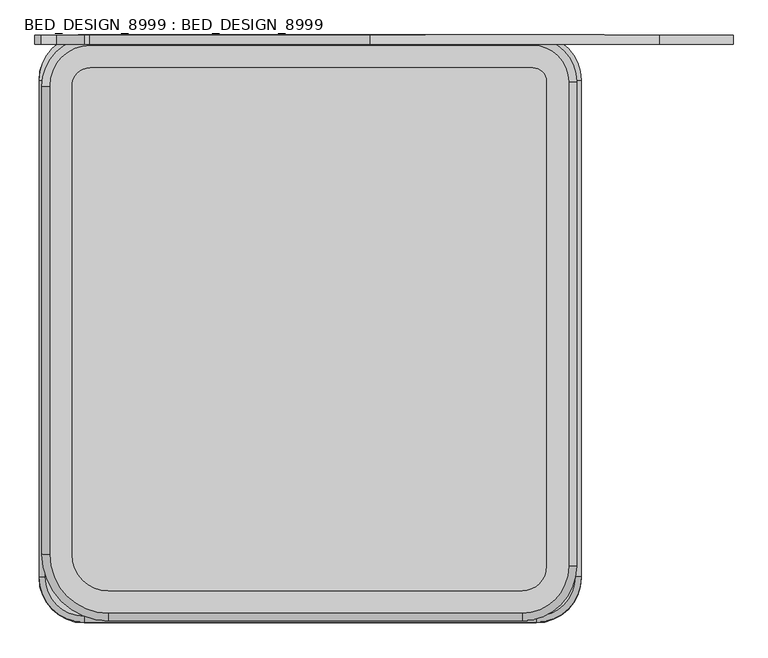
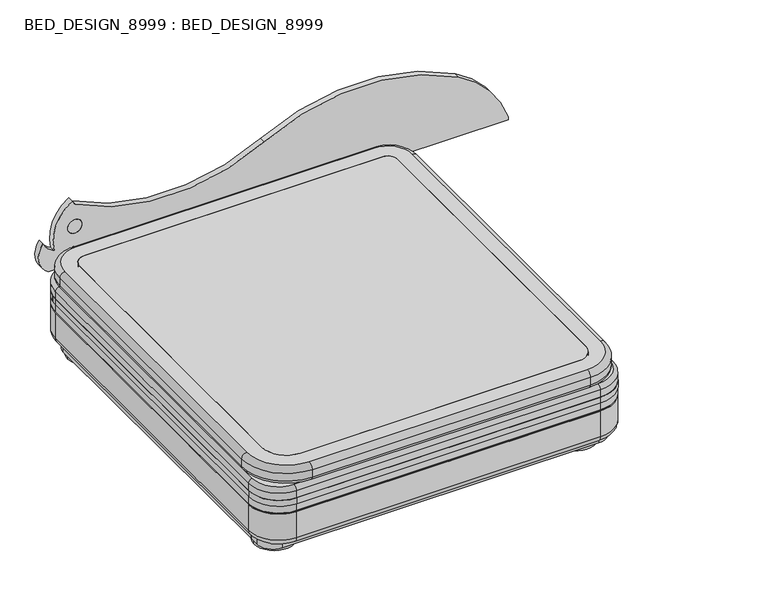
"""IFC4 building model written with IfcOpenShell, lengths in millimetres: furniture geometry, BED_DESIGN_8999 : BED_DESIGN_8999."""

from ifc_helpers import new_model, si_unit, point, frame, frame_2d, origin, origin_with_axes, place, context, project, spatial, polyline, circle_curve, ellipse_curve, trimmed, segment, composite_curve, outline, extrude, source, transform, mapped, element, save
from ifc_brep_helpers import plane_surface, cylinder_surface, revolved_surface, advanced_brep


def bed_design_8999_bed_design_8999_9c973422(model_context):
    return source(origin(), model_context, "Body", "SolidModel", [
        advanced_brep(
        [(550.0, 1945.0, 246.875), (695.0, 1800.0, 246.875), (695.0, 1800.0, 239.375), (550.0, 1945.0, 239.375), (550.0, 1950.0, 350.0), (700.0, 1800.0, 350.0), (700.0, 1800.0, 246.875), (550.0, 1950.0, 246.875), (550.0, 1880.0, 70.0), (630.0, 1800.0, 70.0), (630.0, 1800.0, 370.0), (550.0, 1880.0, 370.0), (550.0, 1950.0, 105.0), (700.0, 1800.0, 105.0), (665.0, 1800.0, 70.0), (550.0, 1915.0, 70.0), (550.0, 1950.0, 239.375), (700.0, 1800.0, 239.375), (-950.0, 1945.0, 239.375), (-950.0, 1945.0, 246.875), (-950.0, 1950.0, 246.875), (-950.0, 1950.0, 350.0), (-950.0, 1880.0, 370.0), (-950.0, 1880.0, 70.0), (-950.0, 1915.0, 70.0), (-950.0, 1950.0, 105.0), (-950.0, 1950.0, 239.375), (-1095.0, 1800.0, 246.875), (-1095.0, 1800.0, 239.375), (-1100.0, 1800.0, 350.0), (-1100.0, 1800.0, 246.875), (-1030.0, 1800.0, 70.0), (-1030.0, 1800.0, 370.0), (-1100.0, 1800.0, 105.0), (-1065.0, 1800.0, 70.0), (-1100.0, 1800.0, 239.375), (-1095.0, 150.0, 239.375), (-1095.0, 150.0, 246.875), (-1100.0, 150.0, 246.875), (-1100.0, 150.0, 350.0), (-1030.0, 150.0, 370.0), (-1030.0, 150.0, 70.0), (-1065.0, 150.0, 70.0), (-1100.0, 150.0, 105.0), (-1100.0, 150.0, 239.375), (-950.0, 5.0, 246.875), (-950.0, 5.0, 239.375), (-950.0, 0.0, 350.0), (-950.0, 0.0, 246.875), (-950.0, 70.0, 70.0), (-950.0, 70.0, 370.0), (-950.0, 0.0, 105.0), (-950.0, 35.0, 70.0), (-950.0, 0.0, 239.375), (550.0, 5.0, 239.375), (550.0, 5.0, 246.875), (550.0, 0.0, 246.875), (550.0, 0.0, 350.0), (550.0, 70.0, 370.0), (550.0, 70.0, 70.0), (550.0, 35.0, 70.0), (550.0, 0.0, 105.0), (550.0, 0.0, 239.375), (695.0, 150.0, 246.875), (695.0, 150.0, 239.375), (700.0, 150.0, 350.0), (700.0, 150.0, 246.875), (630.0, 150.0, 70.0), (630.0, 150.0, 370.0), (700.0, 150.0, 105.0), (665.0, 150.0, 70.0), (700.0, 150.0, 239.375), (-950.0, 20.0, 370.0), (550.0, 20.0, 370.0), (680.0, 150.0, 370.0), (680.0, 1800.0, 370.0), (550.0, 1930.0, 370.0), (-950.0, 1930.0, 370.0), (-1080.0, 1800.0, 370.0), (-1080.0, 150.0, 370.0)],
        [
            (0, 1, circle_curve(frame((550.0, 1800.0, 246.875), z_axis=(0.0, 0.0, -1.0), x_axis=(1.0, 0.0, 0.0)), 145.0)),
            (1, 2),
            (2, 3, circle_curve(frame((550.0, 1800.0, 239.375), z_axis=(0.0, 0.0, 1.0), x_axis=(1.0, 0.0, 0.0)), 145.0)),
            (3, 0),
            (4, 5, circle_curve(frame((550.0, 1800.0, 350.0), z_axis=(0.0, 0.0, -1.0), x_axis=(1.0, 0.0, 0.0)), 150.0)),
            (5, 6),
            (6, 7, circle_curve(frame((550.0, 1800.0, 246.875), z_axis=(0.0, 0.0, 1.0), x_axis=(1.0, 0.0, 0.0)), 150.0)),
            (7, 4),
            (8, 9, circle_curve(frame((550.0, 1800.0, 70.0), z_axis=(0.0, 0.0, -1.0), x_axis=(1.0, 0.0, 0.0)), 80.0)),
            (9, 10),
            (10, 11, circle_curve(frame((550.0, 1800.0, 370.0), z_axis=(0.0, 0.0, 1.0), x_axis=(1.0, 0.0, 0.0)), 80.0)),
            (11, 8),
            (12, 13, circle_curve(frame((550.0, 1800.0, 105.0), z_axis=(0.0, 0.0, -1.0), x_axis=(1.0, 0.0, 0.0)), 150.0)),
            (13, 14, circle_curve(frame((665.0, 1800.0, 105.0), z_axis=(0.0, 1.0, 0.0), x_axis=(1.0, 0.0, 0.0)), 35.0)),
            (14, 15, circle_curve(frame((550.0, 1800.0, 70.0), z_axis=(0.0, 0.0, 1.0), x_axis=(1.0, 0.0, 0.0)), 115.0)),
            (15, 12, circle_curve(frame((550.0, 1915.0, 105.0), z_axis=(1.0, 0.0, 0.0), x_axis=(0.0, 1.0, 0.0)), 35.0)),
            (16, 17, circle_curve(frame((550.0, 1800.0, 239.375), z_axis=(0.0, 0.0, -1.0), x_axis=(1.0, 0.0, 0.0)), 150.0)),
            (17, 13),
            (12, 16),
            (3, 18),
            (18, 19),
            (19, 0),
            (7, 20),
            (20, 21),
            (21, 4),
            (11, 22),
            (22, 23),
            (23, 8),
            (15, 24),
            (24, 25, circle_curve(frame((-950.0, 1915.0, 105.0), z_axis=(1.0, 0.0, 0.0), x_axis=(0.0, 1.0, 0.0)), 35.0)),
            (25, 12),
            (25, 26),
            (26, 16),
            (27, 19, circle_curve(frame((-950.0, 1800.0, 246.875), z_axis=(0.0, 0.0, -1.0), x_axis=(0.0, 1.0, 0.0)), 145.0)),
            (18, 28, circle_curve(frame((-950.0, 1800.0, 239.375), z_axis=(0.0, 0.0, 1.0), x_axis=(0.0, 1.0, 0.0)), 145.0)),
            (28, 27),
            (29, 21, circle_curve(frame((-950.0, 1800.0, 350.0), z_axis=(0.0, 0.0, -1.0), x_axis=(0.0, 1.0, 0.0)), 150.0)),
            (20, 30, circle_curve(frame((-950.0, 1800.0, 246.875), z_axis=(0.0, 0.0, 1.0), x_axis=(0.0, 1.0, 0.0)), 150.0)),
            (30, 29),
            (31, 23, circle_curve(frame((-950.0, 1800.0, 70.0), z_axis=(0.0, 0.0, -1.0), x_axis=(0.0, 1.0, 0.0)), 80.0)),
            (22, 32, circle_curve(frame((-950.0, 1800.0, 370.0), z_axis=(0.0, 0.0, 1.0), x_axis=(0.0, 1.0, 0.0)), 80.0)),
            (32, 31),
            (33, 25, circle_curve(frame((-950.0, 1800.0, 105.0), z_axis=(0.0, 0.0, -1.0), x_axis=(0.0, 1.0, 0.0)), 150.0)),
            (24, 34, circle_curve(frame((-950.0, 1800.0, 70.0), z_axis=(0.0, 0.0, 1.0), x_axis=(0.0, 1.0, 0.0)), 115.0)),
            (34, 33, circle_curve(frame((-1065.0, 1800.0, 105.0), z_axis=(0.0, 1.0, 0.0), x_axis=(-1.0, 0.0, 0.0)), 35.0)),
            (35, 26, circle_curve(frame((-950.0, 1800.0, 239.375), z_axis=(0.0, 0.0, -1.0), x_axis=(0.0, 1.0, 0.0)), 150.0)),
            (33, 35),
            (28, 36),
            (36, 37),
            (37, 27),
            (30, 38),
            (38, 39),
            (39, 29),
            (32, 40),
            (40, 41),
            (41, 31),
            (34, 42),
            (42, 43, circle_curve(frame((-1065.0, 150.0, 105.0), z_axis=(0.0, 1.0, 0.0), x_axis=(-1.0, 0.0, 0.0)), 35.0)),
            (43, 33),
            (43, 44),
            (44, 35),
            (45, 37, circle_curve(frame((-950.0, 150.0, 246.875), z_axis=(0.0, 0.0, -1.0), x_axis=(-1.0, 0.0, 0.0)), 145.0)),
            (36, 46, circle_curve(frame((-950.0, 150.0, 239.375), z_axis=(0.0, 0.0, 1.0), x_axis=(-1.0, 0.0, 0.0)), 145.0)),
            (46, 45),
            (47, 39, circle_curve(frame((-950.0, 150.0, 350.0), z_axis=(0.0, 0.0, -1.0), x_axis=(-1.0, 0.0, 0.0)), 150.0)),
            (38, 48, circle_curve(frame((-950.0, 150.0, 246.875), z_axis=(0.0, 0.0, 1.0), x_axis=(-1.0, 0.0, 0.0)), 150.0)),
            (48, 47),
            (49, 41, circle_curve(frame((-950.0, 150.0, 70.0), z_axis=(0.0, 0.0, -1.0), x_axis=(-1.0, 0.0, 0.0)), 80.0)),
            (40, 50, circle_curve(frame((-950.0, 150.0, 370.0), z_axis=(0.0, 0.0, 1.0), x_axis=(-1.0, 0.0, 0.0)), 80.0)),
            (50, 49),
            (51, 43, circle_curve(frame((-950.0, 150.0, 105.0), z_axis=(0.0, 0.0, -1.0), x_axis=(-1.0, 0.0, 0.0)), 150.0)),
            (42, 52, circle_curve(frame((-950.0, 150.0, 70.0), z_axis=(0.0, 0.0, 1.0), x_axis=(-1.0, 0.0, 0.0)), 115.0)),
            (52, 51, circle_curve(frame((-950.0, 35.0, 105.0), z_axis=(-1.0, 0.0, 0.0), x_axis=(0.0, -1.0, 0.0)), 35.0)),
            (53, 44, circle_curve(frame((-950.0, 150.0, 239.375), z_axis=(0.0, 0.0, -1.0), x_axis=(-1.0, 0.0, 0.0)), 150.0)),
            (51, 53),
            (46, 54),
            (54, 55),
            (55, 45),
            (48, 56),
            (56, 57),
            (57, 47),
            (50, 58),
            (58, 59),
            (59, 49),
            (52, 60),
            (60, 61, circle_curve(frame((550.0, 35.0, 105.0), z_axis=(-1.0, 0.0, 0.0), x_axis=(0.0, -1.0, 0.0)), 35.0)),
            (61, 51),
            (61, 62),
            (62, 53),
            (63, 55, circle_curve(frame((550.0, 150.0, 246.875), z_axis=(0.0, 0.0, -1.0), x_axis=(0.0, -1.0, 0.0)), 145.0)),
            (54, 64, circle_curve(frame((550.0, 150.0, 239.375), z_axis=(0.0, 0.0, 1.0), x_axis=(0.0, -1.0, 0.0)), 145.0)),
            (64, 63),
            (65, 57, circle_curve(frame((550.0, 150.0, 350.0), z_axis=(0.0, 0.0, -1.0), x_axis=(0.0, -1.0, 0.0)), 150.0)),
            (56, 66, circle_curve(frame((550.0, 150.0, 246.875), z_axis=(0.0, 0.0, 1.0), x_axis=(0.0, -1.0, 0.0)), 150.0)),
            (66, 65),
            (67, 59, circle_curve(frame((550.0, 150.0, 70.0), z_axis=(0.0, 0.0, -1.0), x_axis=(0.0, -1.0, 0.0)), 80.0)),
            (58, 68, circle_curve(frame((550.0, 150.0, 370.0), z_axis=(0.0, 0.0, 1.0), x_axis=(0.0, -1.0, 0.0)), 80.0)),
            (68, 67),
            (69, 61, circle_curve(frame((550.0, 150.0, 105.0), z_axis=(0.0, 0.0, -1.0), x_axis=(0.0, -1.0, 0.0)), 150.0)),
            (60, 70, circle_curve(frame((550.0, 150.0, 70.0), z_axis=(0.0, 0.0, 1.0), x_axis=(0.0, -1.0, 0.0)), 115.0)),
            (70, 69, circle_curve(frame((665.0, 150.0, 105.0), z_axis=(0.0, -1.0, 0.0), x_axis=(1.0, 0.0, 0.0)), 35.0)),
            (71, 62, circle_curve(frame((550.0, 150.0, 239.375), z_axis=(0.0, 0.0, -1.0), x_axis=(0.0, -1.0, 0.0)), 150.0)),
            (69, 71),
            (71, 17),
            (2, 64),
            (1, 63),
            (6, 66),
            (5, 65),
            (72, 73),
            (73, 74, circle_curve(frame((550.0, 150.0, 370.0), z_axis=(0.0, 0.0, 1.0), x_axis=(0.0, -1.0, 0.0)), 130.0)),
            (74, 75),
            (75, 76, circle_curve(frame((550.0, 1800.0, 370.0), z_axis=(0.0, 0.0, 1.0), x_axis=(1.0, 0.0, 0.0)), 130.0)),
            (76, 77),
            (77, 78, circle_curve(frame((-950.0, 1800.0, 370.0), z_axis=(0.0, 0.0, 1.0), x_axis=(0.0, 1.0, 0.0)), 130.0)),
            (78, 79),
            (79, 72, circle_curve(frame((-950.0, 150.0, 370.0), z_axis=(0.0, 0.0, 1.0), x_axis=(-1.0, 0.0, 0.0)), 130.0)),
            (10, 68),
            (9, 67),
            (14, 70),
            (13, 69),
            (75, 5, circle_curve(frame((680.0, 1800.0, 350.0), z_axis=(0.0, 1.0, 0.0), x_axis=(1.0, 0.0, 0.0)), 20.0)),
            (4, 76, circle_curve(frame((550.0, 1930.0, 350.0), z_axis=(1.0, 0.0, 0.0), x_axis=(0.0, 1.0, 0.0)), 20.0)),
            (21, 77, circle_curve(frame((-950.0, 1930.0, 350.0), z_axis=(1.0, 0.0, 0.0), x_axis=(0.0, 1.0, 0.0)), 20.0)),
            (29, 78, circle_curve(frame((-1080.0, 1800.0, 350.0), z_axis=(0.0, 1.0, 0.0), x_axis=(-1.0, 0.0, 0.0)), 20.0)),
            (39, 79, circle_curve(frame((-1080.0, 150.0, 350.0), z_axis=(0.0, 1.0, 0.0), x_axis=(-1.0, 0.0, 0.0)), 20.0)),
            (47, 72, circle_curve(frame((-950.0, 20.0, 350.0), z_axis=(-1.0, 0.0, 0.0), x_axis=(0.0, -1.0, 0.0)), 20.0)),
            (57, 73, circle_curve(frame((550.0, 20.0, 350.0), z_axis=(-1.0, 0.0, 0.0), x_axis=(0.0, -1.0, 0.0)), 20.0)),
            (65, 74, circle_curve(frame((680.0, 150.0, 350.0), z_axis=(0.0, -1.0, 0.0), x_axis=(1.0, 0.0, 0.0)), 20.0)),
        ],
        [
            cylinder_surface(frame((550.0, 1800.0, 0.0), z_axis=(0.0, 0.0, 1.0), x_axis=(1.0, 0.0, 0.0)), 145.0),
            cylinder_surface(frame((550.0, 1800.0, 0.0), z_axis=(0.0, 0.0, 1.0), x_axis=(1.0, 0.0, 0.0)), 150.0),
            revolved_surface(polyline([(630.0, 1800.0, 370.0), (630.0, 1800.0, 70.0)]), (550.0, 1800.0, 0.0), (0.0, 0.0, 1.0)),
            revolved_surface(trimmed(ellipse_curve(frame((665.0, 1800.0, 105.0), z_axis=(0.0, -1.0, 0.0), x_axis=(1.0, 0.0, 0.0)), 35.0, 35.0), [point((665.0, 1800.0, 70.0))], [point((700.0, 1800.0, 105.0))], True, "CARTESIAN"), (550.0, 1800.0, 0.0), (0.0, 0.0, 1.0)),
            plane_surface(frame((550.0, 1945.0, 239.375), z_axis=(0.0, 1.0, 0.0), x_axis=(-1.0, 0.0, 0.0))),
            plane_surface(frame((550.0, 1950.0, 246.875), z_axis=(0.0, 1.0, 0.0), x_axis=(-1.0, 0.0, 0.0))),
            plane_surface(frame((550.0, 1880.0, 370.0), z_axis=(0.0, -1.0, 0.0), x_axis=(-1.0, 0.0, 0.0))),
            cylinder_surface(frame((550.0, 1915.0, 105.0), z_axis=(1.0, 0.0, 0.0), x_axis=(0.0, 1.0, 0.0)), 35.0),
            plane_surface(frame((550.0, 1950.0, 105.0), z_axis=(0.0, 1.0, 0.0), x_axis=(-1.0, 0.0, 0.0))),
            cylinder_surface(frame((-950.0, 1800.0, 0.0), z_axis=(0.0, 0.0, 1.0), x_axis=(0.0, 1.0, 0.0)), 145.0),
            cylinder_surface(frame((-950.0, 1800.0, 0.0), z_axis=(0.0, 0.0, 1.0), x_axis=(0.0, 1.0, 0.0)), 150.0),
            revolved_surface(polyline([(-950.0, 1880.0, 370.0), (-950.0, 1880.0, 70.0)]), (-950.0, 1800.0, 0.0), (0.0, 0.0, 1.0)),
            revolved_surface(trimmed(ellipse_curve(frame((-950.0, 1915.0, 105.0), z_axis=(1.0, 0.0, 0.0), x_axis=(0.0, 1.0, 0.0)), 35.0, 35.0), [point((-950.0, 1915.0, 70.0))], [point((-950.0, 1950.0, 105.0))], True, "CARTESIAN"), (-950.0, 1800.0, 0.0), (0.0, 0.0, 1.0)),
            plane_surface(frame((-1095.0, 1800.0, 239.375), z_axis=(-1.0, 0.0, 0.0), x_axis=(0.0, -1.0, 0.0))),
            plane_surface(frame((-1100.0, 1800.0, 246.875), z_axis=(-1.0, 0.0, 0.0), x_axis=(0.0, -1.0, 0.0))),
            plane_surface(frame((-1030.0, 1800.0, 370.0), z_axis=(1.0, 0.0, 0.0), x_axis=(0.0, -1.0, 0.0))),
            cylinder_surface(frame((-1065.0, 1800.0, 105.0), z_axis=(0.0, 1.0, 0.0), x_axis=(-1.0, 0.0, 0.0)), 35.0),
            plane_surface(frame((-1100.0, 1800.0, 105.0), z_axis=(-1.0, 0.0, 0.0), x_axis=(0.0, -1.0, 0.0))),
            cylinder_surface(frame((-950.0, 150.0, 0.0), z_axis=(0.0, 0.0, 1.0), x_axis=(-1.0, 0.0, 0.0)), 145.0),
            cylinder_surface(frame((-950.0, 150.0, 0.0), z_axis=(0.0, 0.0, 1.0), x_axis=(-1.0, 0.0, 0.0)), 150.0),
            revolved_surface(polyline([(-1030.0, 150.0, 370.0), (-1030.0, 150.0, 70.0)]), (-950.0, 150.0, 0.0), (0.0, 0.0, 1.0)),
            revolved_surface(trimmed(ellipse_curve(frame((-1065.0, 150.0, 105.0), z_axis=(0.0, 1.0, 0.0), x_axis=(-1.0, 0.0, 0.0)), 35.0, 35.0), [point((-1065.0, 150.0, 70.0))], [point((-1100.0, 150.0, 105.0))], True, "CARTESIAN"), (-950.0, 150.0, 0.0), (0.0, 0.0, 1.0)),
            plane_surface(frame((-950.0, 5.0, 239.375), z_axis=(0.0, -1.0, 0.0), x_axis=(1.0, 0.0, 0.0))),
            plane_surface(frame((-950.0, 0.0, 246.875), z_axis=(0.0, -1.0, 0.0), x_axis=(1.0, 0.0, 0.0))),
            plane_surface(frame((-950.0, 70.0, 370.0), z_axis=(0.0, 1.0, 0.0), x_axis=(1.0, 0.0, 0.0))),
            cylinder_surface(frame((-950.0, 35.0, 105.0), z_axis=(-1.0, 0.0, 0.0), x_axis=(0.0, -1.0, 0.0)), 35.0),
            plane_surface(frame((-950.0, 0.0, 105.0), z_axis=(0.0, -1.0, 0.0), x_axis=(1.0, 0.0, 0.0))),
            cylinder_surface(frame((550.0, 150.0, 0.0), z_axis=(0.0, 0.0, 1.0), x_axis=(0.0, -1.0, 0.0)), 145.0),
            cylinder_surface(frame((550.0, 150.0, 0.0), z_axis=(0.0, 0.0, 1.0), x_axis=(0.0, -1.0, 0.0)), 150.0),
            revolved_surface(polyline([(550.0, 70.0, 370.0), (550.0, 70.0, 70.0)]), (550.0, 150.0, 0.0), (0.0, 0.0, 1.0)),
            revolved_surface(trimmed(ellipse_curve(frame((550.0, 35.0, 105.0), z_axis=(-1.0, 0.0, 0.0), x_axis=(0.0, -1.0, 0.0)), 35.0, 35.0), [point((550.0, 35.0, 70.0))], [point((550.0, 0.0, 105.0))], True, "CARTESIAN"), (550.0, 150.0, 0.0), (0.0, 0.0, 1.0)),
            plane_surface(frame((700.0, 150.0, 239.375), z_axis=(0.0, 0.0, 1.0), x_axis=(0.0, 1.0, 0.0))),
            plane_surface(frame((695.0, 150.0, 239.375), z_axis=(1.0, 0.0, 0.0), x_axis=(0.0, 1.0, 0.0))),
            plane_surface(frame((695.0, 150.0, 246.875), z_axis=(0.0, 0.0, -1.0), x_axis=(0.0, 1.0, 0.0))),
            plane_surface(frame((700.0, 150.0, 246.875), z_axis=(1.0, 0.0, 0.0), x_axis=(0.0, 1.0, 0.0))),
            plane_surface(frame((680.0, 150.0, 370.0), z_axis=(0.0, 0.0, 1.0), x_axis=(0.0, 1.0, 0.0))),
            plane_surface(frame((630.0, 150.0, 370.0), z_axis=(-1.0, 0.0, 0.0), x_axis=(0.0, 1.0, 0.0))),
            plane_surface(frame((630.0, 150.0, 70.0), z_axis=(0.0, 0.0, -1.0), x_axis=(0.0, 1.0, 0.0))),
            cylinder_surface(frame((665.0, 150.0, 105.0), z_axis=(0.0, -1.0, 0.0), x_axis=(1.0, 0.0, 0.0)), 35.0),
            plane_surface(frame((700.0, 150.0, 105.0), z_axis=(1.0, 0.0, 0.0), x_axis=(0.0, 1.0, 0.0))),
            revolved_surface(trimmed(ellipse_curve(frame((680.0, 1800.0, 350.0), z_axis=(0.0, -1.0, 0.0), x_axis=(1.0, 0.0, 0.0)), 20.0, 20.0), [point((700.0, 1800.0, 350.0))], [point((680.0, 1800.0, 370.0))], True, "CARTESIAN"), (550.0, 1800.0, 0.0), (0.0, 0.0, 1.0)),
            cylinder_surface(frame((550.0, 1930.0, 350.0), z_axis=(1.0, 0.0, 0.0), x_axis=(0.0, 1.0, 0.0)), 20.0),
            revolved_surface(trimmed(ellipse_curve(frame((-950.0, 1930.0, 350.0), z_axis=(1.0, 0.0, 0.0), x_axis=(0.0, 1.0, 0.0)), 20.0, 20.0), [point((-950.0, 1950.0, 350.0))], [point((-950.0, 1930.0, 370.0))], True, "CARTESIAN"), (-950.0, 1800.0, 0.0), (0.0, 0.0, 1.0)),
            cylinder_surface(frame((-1080.0, 1800.0, 350.0), z_axis=(0.0, 1.0, 0.0), x_axis=(-1.0, 0.0, 0.0)), 20.0),
            revolved_surface(trimmed(ellipse_curve(frame((-1080.0, 150.0, 350.0), z_axis=(0.0, 1.0, 0.0), x_axis=(-1.0, 0.0, 0.0)), 20.0, 20.0), [point((-1100.0, 150.0, 350.0))], [point((-1080.0, 150.0, 370.0))], True, "CARTESIAN"), (-950.0, 150.0, 0.0), (0.0, 0.0, 1.0)),
            cylinder_surface(frame((-950.0, 20.0, 350.0), z_axis=(-1.0, 0.0, 0.0), x_axis=(0.0, -1.0, 0.0)), 20.0),
            revolved_surface(trimmed(ellipse_curve(frame((550.0, 20.0, 350.0), z_axis=(-1.0, 0.0, 0.0), x_axis=(0.0, -1.0, 0.0)), 20.0, 20.0), [point((550.0, 0.0, 350.0))], [point((550.0, 20.0, 370.0))], True, "CARTESIAN"), (550.0, 150.0, 0.0), (0.0, 0.0, 1.0)),
            cylinder_surface(frame((680.0, 150.0, 350.0), z_axis=(0.0, -1.0, 0.0), x_axis=(1.0, 0.0, 0.0)), 20.0),
        ],
        [
            (0, [[1, 2, 3, 4]]),
            (1, [[5, 6, 7, 8]]),
            (2, [[9, 10, 11, 12]]),
            (3, [[13, 14, 15, 16]]),
            (1, [[17, 18, -13, 19]]),
            (4, [[-4, 20, 21, 22]]),
            (5, [[-8, 23, 24, 25]]),
            (6, [[-12, 26, 27, 28]]),
            (7, [[-16, 29, 30, 31]]),
            (8, [[-19, -31, 32, 33]]),
            (9, [[34, -21, 35, 36]]),
            (10, [[37, -24, 38, 39]]),
            (11, [[40, -27, 41, 42]]),
            (12, [[43, -30, 44, 45]]),
            (10, [[46, -32, -43, 47]]),
            (13, [[-36, 48, 49, 50]]),
            (14, [[-39, 51, 52, 53]]),
            (15, [[-42, 54, 55, 56]]),
            (16, [[-45, 57, 58, 59]]),
            (17, [[-47, -59, 60, 61]]),
            (18, [[62, -49, 63, 64]]),
            (19, [[65, -52, 66, 67]]),
            (20, [[68, -55, 69, 70]]),
            (21, [[71, -58, 72, 73]]),
            (19, [[74, -60, -71, 75]]),
            (22, [[-64, 76, 77, 78]]),
            (23, [[-67, 79, 80, 81]]),
            (24, [[-70, 82, 83, 84]]),
            (25, [[-73, 85, 86, 87]]),
            (26, [[-75, -87, 88, 89]]),
            (27, [[90, -77, 91, 92]]),
            (28, [[93, -80, 94, 95]]),
            (29, [[96, -83, 97, 98]]),
            (30, [[99, -86, 100, 101]]),
            (28, [[102, -88, -99, 103]]),
            (31, [[-89, -102, 104, -17, -33, -46, -61, -74], [105, -91, -76, -63, -48, -35, -20, -3]]),
            (32, [[-92, -105, -2, 106]]),
            (33, [[107, -94, -79, -66, -51, -38, -23, -7], [-78, -90, -106, -1, -22, -34, -50, -62]]),
            (34, [[-95, -107, -6, 108]]),
            (35, [[109, 110, 111, 112, 113, 114, 115, 116], [117, -97, -82, -69, -54, -41, -26, -11]]),
            (36, [[-98, -117, -10, 118]]),
            (37, [[119, -100, -85, -72, -57, -44, -29, -15], [-84, -96, -118, -9, -28, -40, -56, -68]]),
            (38, [[-101, -119, -14, 120]]),
            (39, [[-103, -120, -18, -104]]),
            (40, [[-112, 121, -5, 122]]),
            (41, [[-122, -25, 123, -113]]),
            (42, [[-114, -123, -37, 124]]),
            (43, [[-124, -53, 125, -115]]),
            (44, [[-116, -125, -65, 126]]),
            (45, [[-126, -81, 127, -109]]),
            (46, [[-110, -127, -93, 128]]),
            (47, [[-128, -108, -121, -111]]),
        ],
    ),
        extrude(outline(composite_curve([segment(trimmed(circle_curve(frame_2d((583.4768071, 1800.0)), 80.0), [point((583.4768071, 1880.0))], [point((663.4768071, 1800.0))], False, "CARTESIAN"), True, "CONTINUOUS"), segment(polyline([(663.4768071, 1800.0), (663.4768071, 150.0)]), True, "CONTINUOUS"), segment(trimmed(circle_curve(frame_2d((583.4768071, 150.0)), 80.0), [point((663.4768071, 150.0))], [point((583.4768071, 70.0))], False, "CARTESIAN"), True, "CONTINUOUS"), segment(polyline([(583.4768071, 70.0), (-980.0, 70.0)]), True, "CONTINUOUS"), segment(trimmed(circle_curve(frame_2d((-980.0, 150.0)), 80.0), [point((-980.0, 70.0))], [point((-1060.0, 150.0))], False, "CARTESIAN"), True, "CONTINUOUS"), segment(polyline([(-1060.0, 150.0), (-1060.0, 1800.0)]), True, "CONTINUOUS"), segment(trimmed(circle_curve(frame_2d((-980.0, 1800.0)), 80.0), [point((-1060.0, 1800.0))], [point((-980.0, 1880.0))], False, "CARTESIAN"), True, "CONTINUOUS"), segment(polyline([(-980.0, 1880.0), (583.4768071, 1880.0)]), True, "CONTINUOUS")], self_intersect=False)), frame((0.0, 0.0, 20.0), z_axis=(0.0, 0.0, 1.0), x_axis=(1.0, 0.0, 0.0)), (0.0, 0.0, 1.0), 50.0),
        extrude(outline(composite_curve([segment(polyline([(550.3311653, -2.3890651), (-950.4866101, -2.3890651)]), True, "CONTINUOUS"), segment(trimmed(circle_curve(frame_2d((-950.4866101, 147.6109349)), 150.0), [point((-950.4866101, -2.3890651))], [point((-1100.4866101, 147.6109349))], False, "CARTESIAN"), True, "CONTINUOUS"), segment(polyline([(-1100.4866101, 147.6109349), (-1100.4866101, 1800.1750141)]), True, "CONTINUOUS"), segment(trimmed(circle_curve(frame_2d((-950.4866101, 1800.1750141)), 150.0), [point((-1100.4866101, 1800.1750141))], [point((-950.4866101, 1950.1750141))], False, "CARTESIAN"), True, "CONTINUOUS"), segment(polyline([(-950.4866101, 1950.1750141), (550.3311653, 1950.1750141)]), True, "CONTINUOUS"), segment(trimmed(circle_curve(frame_2d((550.3311653, 1800.1750141)), 150.0), [point((550.3311653, 1950.1750141))], [point((700.3311653, 1800.1750141))], False, "CARTESIAN"), True, "CONTINUOUS"), segment(polyline([(700.3311653, 1800.1750141), (700.3311653, 147.6109349)]), True, "CONTINUOUS"), segment(trimmed(circle_curve(frame_2d((550.3311653, 147.6109349)), 150.0), [point((700.3311653, 147.6109349))], [point((550.3311653, -2.3890651))], False, "CARTESIAN"), True, "CONTINUOUS")], self_intersect=False)), frame((0.0, 0.0, 283.4375), z_axis=(0.0, 0.0, 1.0), x_axis=(1.0, 0.0, 0.0)), (0.0, 0.0, 1.0), 30.0),
        advanced_brep(
        [(538.4768071, 1915.890134, 454.4796821), (659.3669411, 1795.0, 454.4796821), (684.3669411, 1795.0, 429.4796821), (538.4768071, 1940.890134, 429.4796821), (538.4768071, 1840.890134, 369.4796821), (584.3669411, 1795.0, 369.4796821), (584.3669411, 1795.0, 454.4796821), (538.4768071, 1840.890134, 454.4796821), (538.4768071, 1940.890134, 389.4796821), (684.3669411, 1795.0, 389.4796821), (664.3669411, 1795.0, 369.4796821), (538.4768071, 1920.890134, 369.4796821), (-930.0, 1940.890134, 429.4796821), (-930.0, 1915.890134, 454.4796821), (-930.0, 1840.890134, 454.4796821), (-930.0, 1840.890134, 369.4796821), (-930.0, 1920.890134, 369.4796821), (-930.0, 1940.890134, 389.4796821), (-1065.890134, 1780.0, 454.4796821), (-1090.890134, 1780.0, 429.4796821), (-990.890134, 1780.0, 369.4796821), (-990.890134, 1780.0, 454.4796821), (-1090.890134, 1780.0, 389.4796821), (-1070.890134, 1780.0, 369.4796821), (-1090.890134, 225.0, 429.4796821), (-1065.890134, 225.0, 454.4796821), (-990.890134, 225.0, 454.4796821), (-990.890134, 225.0, 369.4796821), (-1070.890134, 225.0, 369.4796821), (-1090.890134, 225.0, 389.4796821), (-870.0, 29.109866, 454.4796821), (-870.0, 4.109866, 429.4796821), (-870.0, 104.109866, 369.4796821), (-870.0, 104.109866, 454.4796821), (-870.0, 4.109866, 389.4796821), (-870.0, 24.109866, 369.4796821), (503.4768071, 4.109866, 429.4796821), (503.4768071, 29.109866, 454.4796821), (503.4768071, 104.109866, 454.4796821), (503.4768071, 104.109866, 369.4796821), (503.4768071, 24.109866, 369.4796821), (503.4768071, 4.109866, 389.4796821), (659.3669411, 185.0, 454.4796821), (684.3669411, 185.0, 429.4796821), (584.3669411, 185.0, 369.4796821), (584.3669411, 185.0, 454.4796821), (684.3669411, 185.0, 389.4796821), (664.3669411, 185.0, 369.4796821)],
        [
            (0, 1, circle_curve(frame((538.4768071, 1795.0, 454.4796821), z_axis=(0.0, 0.0, -1.0), x_axis=(1.0, 0.0, 0.0)), 120.890134)),
            (1, 2, circle_curve(frame((659.3669411, 1795.0, 429.4796821), z_axis=(0.0, 1.0, 0.0), x_axis=(1.0, 0.0, 0.0)), 25.0)),
            (2, 3, circle_curve(frame((538.4768071, 1795.0, 429.4796821), z_axis=(0.0, 0.0, 1.0), x_axis=(1.0, 0.0, 0.0)), 145.890134)),
            (3, 0, circle_curve(frame((538.4768071, 1915.890134, 429.4796821), z_axis=(1.0, 0.0, 0.0), x_axis=(0.0, 1.0, 0.0)), 25.0)),
            (4, 5, circle_curve(frame((538.4768071, 1795.0, 369.4796821), z_axis=(0.0, 0.0, -1.0), x_axis=(1.0, 0.0, 0.0)), 45.890134)),
            (5, 6),
            (6, 7, circle_curve(frame((538.4768071, 1795.0, 454.4796821), z_axis=(0.0, 0.0, 1.0), x_axis=(1.0, 0.0, 0.0)), 45.890134)),
            (7, 4),
            (8, 9, circle_curve(frame((538.4768071, 1795.0, 389.4796821), z_axis=(0.0, 0.0, -1.0), x_axis=(1.0, 0.0, 0.0)), 145.890134)),
            (9, 10, circle_curve(frame((664.3669411, 1795.0, 389.4796821), z_axis=(0.0, 1.0, 0.0), x_axis=(1.0, 0.0, 0.0)), 20.0)),
            (10, 11, circle_curve(frame((538.4768071, 1795.0, 369.4796821), z_axis=(0.0, 0.0, 1.0), x_axis=(1.0, 0.0, 0.0)), 125.890134)),
            (11, 8, circle_curve(frame((538.4768071, 1920.890134, 389.4796821), z_axis=(1.0, 0.0, 0.0), x_axis=(0.0, 1.0, 0.0)), 20.0)),
            (2, 9),
            (8, 3),
            (3, 12),
            (12, 13, circle_curve(frame((-930.0, 1915.890134, 429.4796821), z_axis=(1.0, 0.0, 0.0), x_axis=(0.0, 1.0, 0.0)), 25.0)),
            (13, 0),
            (7, 14),
            (14, 15),
            (15, 4),
            (11, 16),
            (16, 17, circle_curve(frame((-930.0, 1920.890134, 389.4796821), z_axis=(1.0, 0.0, 0.0), x_axis=(0.0, 1.0, 0.0)), 20.0)),
            (17, 8),
            (17, 12),
            (18, 13, circle_curve(frame((-930.0, 1780.0, 454.4796821), z_axis=(0.0, 0.0, -1.0), x_axis=(0.0, 1.0, 0.0)), 135.890134)),
            (12, 19, circle_curve(frame((-930.0, 1780.0, 429.4796821), z_axis=(0.0, 0.0, 1.0), x_axis=(0.0, 1.0, 0.0)), 160.890134)),
            (19, 18, circle_curve(frame((-1065.890134, 1780.0, 429.4796821), z_axis=(0.0, 1.0, 0.0), x_axis=(-1.0, 0.0, 0.0)), 25.0)),
            (20, 15, circle_curve(frame((-930.0, 1780.0, 369.4796821), z_axis=(0.0, 0.0, -1.0), x_axis=(0.0, 1.0, 0.0)), 60.890134)),
            (14, 21, circle_curve(frame((-930.0, 1780.0, 454.4796821), z_axis=(0.0, 0.0, 1.0), x_axis=(0.0, 1.0, 0.0)), 60.890134)),
            (21, 20),
            (22, 17, circle_curve(frame((-930.0, 1780.0, 389.4796821), z_axis=(0.0, 0.0, -1.0), x_axis=(0.0, 1.0, 0.0)), 160.890134)),
            (16, 23, circle_curve(frame((-930.0, 1780.0, 369.4796821), z_axis=(0.0, 0.0, 1.0), x_axis=(0.0, 1.0, 0.0)), 140.890134)),
            (23, 22, circle_curve(frame((-1070.890134, 1780.0, 389.4796821), z_axis=(0.0, 1.0, 0.0), x_axis=(-1.0, 0.0, 0.0)), 20.0)),
            (22, 19),
            (19, 24),
            (24, 25, circle_curve(frame((-1065.890134, 225.0, 429.4796821), z_axis=(0.0, 1.0, 0.0), x_axis=(-1.0, 0.0, 0.0)), 25.0)),
            (25, 18),
            (21, 26),
            (26, 27),
            (27, 20),
            (23, 28),
            (28, 29, circle_curve(frame((-1070.890134, 225.0, 389.4796821), z_axis=(0.0, 1.0, 0.0), x_axis=(-1.0, 0.0, 0.0)), 20.0)),
            (29, 22),
            (29, 24),
            (30, 25, circle_curve(frame((-870.0, 225.0, 454.4796821), z_axis=(0.0, 0.0, -1.0), x_axis=(-1.0, 0.0, 0.0)), 195.890134)),
            (24, 31, circle_curve(frame((-870.0, 225.0, 429.4796821), z_axis=(0.0, 0.0, 1.0), x_axis=(-1.0, 0.0, 0.0)), 220.890134)),
            (31, 30, circle_curve(frame((-870.0, 29.109866, 429.4796821), z_axis=(-1.0, 0.0, 0.0), x_axis=(0.0, -1.0, 0.0)), 25.0)),
            (32, 27, circle_curve(frame((-870.0, 225.0, 369.4796821), z_axis=(0.0, 0.0, -1.0), x_axis=(-1.0, 0.0, 0.0)), 120.890134)),
            (26, 33, circle_curve(frame((-870.0, 225.0, 454.4796821), z_axis=(0.0, 0.0, 1.0), x_axis=(-1.0, 0.0, 0.0)), 120.890134)),
            (33, 32),
            (34, 29, circle_curve(frame((-870.0, 225.0, 389.4796821), z_axis=(0.0, 0.0, -1.0), x_axis=(-1.0, 0.0, 0.0)), 220.890134)),
            (28, 35, circle_curve(frame((-870.0, 225.0, 369.4796821), z_axis=(0.0, 0.0, 1.0), x_axis=(-1.0, 0.0, 0.0)), 200.890134)),
            (35, 34, circle_curve(frame((-870.0, 24.109866, 389.4796821), z_axis=(-1.0, 0.0, 0.0), x_axis=(0.0, -1.0, 0.0)), 20.0)),
            (34, 31),
            (31, 36),
            (36, 37, circle_curve(frame((503.4768071, 29.109866, 429.4796821), z_axis=(-1.0, 0.0, 0.0), x_axis=(0.0, -1.0, 0.0)), 25.0)),
            (37, 30),
            (33, 38),
            (38, 39),
            (39, 32),
            (35, 40),
            (40, 41, circle_curve(frame((503.4768071, 24.109866, 389.4796821), z_axis=(-1.0, 0.0, 0.0), x_axis=(0.0, -1.0, 0.0)), 20.0)),
            (41, 34),
            (41, 36),
            (42, 37, circle_curve(frame((503.4768071, 185.0, 454.4796821), z_axis=(0.0, 0.0, -1.0), x_axis=(0.0, -1.0, 0.0)), 155.890134)),
            (36, 43, circle_curve(frame((503.4768071, 185.0, 429.4796821), z_axis=(0.0, 0.0, 1.0), x_axis=(0.0, -1.0, 0.0)), 180.890134)),
            (43, 42, circle_curve(frame((659.3669411, 185.0, 429.4796821), z_axis=(0.0, -1.0, 0.0), x_axis=(1.0, 0.0, 0.0)), 25.0)),
            (44, 39, circle_curve(frame((503.4768071, 185.0, 369.4796821), z_axis=(0.0, 0.0, -1.0), x_axis=(0.0, -1.0, 0.0)), 80.890134)),
            (38, 45, circle_curve(frame((503.4768071, 185.0, 454.4796821), z_axis=(0.0, 0.0, 1.0), x_axis=(0.0, -1.0, 0.0)), 80.890134)),
            (45, 44),
            (46, 41, circle_curve(frame((503.4768071, 185.0, 389.4796821), z_axis=(0.0, 0.0, -1.0), x_axis=(0.0, -1.0, 0.0)), 180.890134)),
            (40, 47, circle_curve(frame((503.4768071, 185.0, 369.4796821), z_axis=(0.0, 0.0, 1.0), x_axis=(0.0, -1.0, 0.0)), 160.890134)),
            (47, 46, circle_curve(frame((664.3669411, 185.0, 389.4796821), z_axis=(0.0, -1.0, 0.0), x_axis=(1.0, 0.0, 0.0)), 20.0)),
            (46, 43),
            (43, 2),
            (1, 42),
            (6, 45),
            (5, 44),
            (10, 47),
            (9, 46),
        ],
        [
            revolved_surface(trimmed(ellipse_curve(frame((659.3669411, 1795.0, 429.4796821), z_axis=(0.0, -1.0, 0.0), x_axis=(1.0, 0.0, 0.0)), 25.0, 25.0), [point((684.3669411, 1795.0, 429.4796821))], [point((659.3669411, 1795.0, 454.4796821))], True, "CARTESIAN"), (538.4768071, 1795.0, 0.0), (0.0, 0.0, 1.0)),
            revolved_surface(polyline([(584.3669411, 1795.0, 454.4796821), (584.3669411, 1795.0, 369.4796821)]), (538.4768071, 1795.0, 0.0), (0.0, 0.0, 1.0)),
            revolved_surface(trimmed(ellipse_curve(frame((664.3669411, 1795.0, 389.4796821), z_axis=(0.0, -1.0, 0.0), x_axis=(1.0, 0.0, 0.0)), 20.0, 20.0), [point((664.3669411, 1795.0, 369.4796821))], [point((684.3669411, 1795.0, 389.4796821))], True, "CARTESIAN"), (538.4768071, 1795.0, 0.0), (0.0, 0.0, 1.0)),
            cylinder_surface(frame((538.4768071, 1795.0, 0.0), z_axis=(0.0, 0.0, 1.0), x_axis=(1.0, 0.0, 0.0)), 145.890134),
            cylinder_surface(frame((538.4768071, 1915.890134, 429.4796821), z_axis=(1.0, 0.0, 0.0), x_axis=(0.0, 1.0, 0.0)), 25.0),
            plane_surface(frame((538.4768071, 1840.890134, 454.4796821), z_axis=(0.0, -1.0, 0.0), x_axis=(-1.0, 0.0, 0.0))),
            cylinder_surface(frame((538.4768071, 1920.890134, 389.4796821), z_axis=(1.0, 0.0, 0.0), x_axis=(0.0, 1.0, 0.0)), 20.0),
            plane_surface(frame((538.4768071, 1940.890134, 389.4796821), z_axis=(0.0, 1.0, 0.0), x_axis=(-1.0, 0.0, 0.0))),
            revolved_surface(trimmed(ellipse_curve(frame((-930.0, 1915.890134, 429.4796821), z_axis=(1.0, 0.0, 0.0), x_axis=(0.0, 1.0, 0.0)), 25.0, 25.0), [point((-930.0, 1940.890134, 429.4796821))], [point((-930.0, 1915.890134, 454.4796821))], True, "CARTESIAN"), (-930.0, 1780.0, 0.0), (0.0, 0.0, 1.0)),
            revolved_surface(polyline([(-930.0, 1840.890134, 454.4796821), (-930.0, 1840.890134, 369.4796821)]), (-930.0, 1780.0, 0.0), (0.0, 0.0, 1.0)),
            revolved_surface(trimmed(ellipse_curve(frame((-930.0, 1920.890134, 389.4796821), z_axis=(1.0, 0.0, 0.0), x_axis=(0.0, 1.0, 0.0)), 20.0, 20.0), [point((-930.0, 1920.890134, 369.4796821))], [point((-930.0, 1940.890134, 389.4796821))], True, "CARTESIAN"), (-930.0, 1780.0, 0.0), (0.0, 0.0, 1.0)),
            cylinder_surface(frame((-930.0, 1780.0, 0.0), z_axis=(0.0, 0.0, 1.0), x_axis=(0.0, 1.0, 0.0)), 160.890134),
            cylinder_surface(frame((-1065.890134, 1780.0, 429.4796821), z_axis=(0.0, 1.0, 0.0), x_axis=(-1.0, 0.0, 0.0)), 25.0),
            plane_surface(frame((-990.890134, 1780.0, 454.4796821), z_axis=(1.0, 0.0, 0.0), x_axis=(0.0, -1.0, 0.0))),
            cylinder_surface(frame((-1070.890134, 1780.0, 389.4796821), z_axis=(0.0, 1.0, 0.0), x_axis=(-1.0, 0.0, 0.0)), 20.0),
            plane_surface(frame((-1090.890134, 1780.0, 389.4796821), z_axis=(-1.0, 0.0, 0.0), x_axis=(0.0, -1.0, 0.0))),
            revolved_surface(trimmed(ellipse_curve(frame((-1065.890134, 225.0, 429.4796821), z_axis=(0.0, 1.0, 0.0), x_axis=(-1.0, 0.0, 0.0)), 25.0, 25.0), [point((-1090.890134, 225.0, 429.4796821))], [point((-1065.890134, 225.0, 454.4796821))], True, "CARTESIAN"), (-870.0, 225.0, 0.0), (0.0, 0.0, 1.0)),
            revolved_surface(polyline([(-990.890134, 225.0, 454.4796821), (-990.890134, 225.0, 369.4796821)]), (-870.0, 225.0, 0.0), (0.0, 0.0, 1.0)),
            revolved_surface(trimmed(ellipse_curve(frame((-1070.890134, 225.0, 389.4796821), z_axis=(0.0, 1.0, 0.0), x_axis=(-1.0, 0.0, 0.0)), 20.0, 20.0), [point((-1070.890134, 225.0, 369.4796821))], [point((-1090.890134, 225.0, 389.4796821))], True, "CARTESIAN"), (-870.0, 225.0, 0.0), (0.0, 0.0, 1.0)),
            cylinder_surface(frame((-870.0, 225.0, 0.0), z_axis=(0.0, 0.0, 1.0), x_axis=(-1.0, 0.0, 0.0)), 220.890134),
            cylinder_surface(frame((-870.0, 29.109866, 429.4796821), z_axis=(-1.0, 0.0, 0.0), x_axis=(0.0, -1.0, 0.0)), 25.0),
            plane_surface(frame((-870.0, 104.109866, 454.4796821), z_axis=(0.0, 1.0, 0.0), x_axis=(1.0, 0.0, 0.0))),
            cylinder_surface(frame((-870.0, 24.109866, 389.4796821), z_axis=(-1.0, 0.0, 0.0), x_axis=(0.0, -1.0, 0.0)), 20.0),
            plane_surface(frame((-870.0, 4.109866, 389.4796821), z_axis=(0.0, -1.0, 0.0), x_axis=(1.0, 0.0, 0.0))),
            revolved_surface(trimmed(ellipse_curve(frame((503.4768071, 29.109866, 429.4796821), z_axis=(-1.0, 0.0, 0.0), x_axis=(0.0, -1.0, 0.0)), 25.0, 25.0), [point((503.4768071, 4.109866, 429.4796821))], [point((503.4768071, 29.109866, 454.4796821))], True, "CARTESIAN"), (503.4768071, 185.0, 0.0), (0.0, 0.0, 1.0)),
            revolved_surface(polyline([(503.4768071, 104.109866, 454.4796821), (503.4768071, 104.109866, 369.4796821)]), (503.4768071, 185.0, 0.0), (0.0, 0.0, 1.0)),
            revolved_surface(trimmed(ellipse_curve(frame((503.4768071, 24.109866, 389.4796821), z_axis=(-1.0, 0.0, 0.0), x_axis=(0.0, -1.0, 0.0)), 20.0, 20.0), [point((503.4768071, 24.109866, 369.4796821))], [point((503.4768071, 4.109866, 389.4796821))], True, "CARTESIAN"), (503.4768071, 185.0, 0.0), (0.0, 0.0, 1.0)),
            cylinder_surface(frame((503.4768071, 185.0, 0.0), z_axis=(0.0, 0.0, 1.0), x_axis=(0.0, -1.0, 0.0)), 180.890134),
            cylinder_surface(frame((659.3669411, 185.0, 429.4796821), z_axis=(0.0, -1.0, 0.0), x_axis=(1.0, 0.0, 0.0)), 25.0),
            plane_surface(frame((659.3669411, 185.0, 454.4796821), z_axis=(0.0, 0.0, 1.0), x_axis=(0.0, 1.0, 0.0))),
            plane_surface(frame((584.3669411, 185.0, 454.4796821), z_axis=(-1.0, 0.0, 0.0), x_axis=(0.0, 1.0, 0.0))),
            plane_surface(frame((584.3669411, 185.0, 369.4796821), z_axis=(0.0, 0.0, -1.0), x_axis=(0.0, 1.0, 0.0))),
            cylinder_surface(frame((664.3669411, 185.0, 389.4796821), z_axis=(0.0, -1.0, 0.0), x_axis=(1.0, 0.0, 0.0)), 20.0),
            plane_surface(frame((684.3669411, 185.0, 389.4796821), z_axis=(1.0, 0.0, 0.0), x_axis=(0.0, 1.0, 0.0))),
        ],
        [
            (0, [[1, 2, 3, 4]]),
            (1, [[5, 6, 7, 8]]),
            (2, [[9, 10, 11, 12]]),
            (3, [[-3, 13, -9, 14]]),
            (4, [[-4, 15, 16, 17]]),
            (5, [[-8, 18, 19, 20]]),
            (6, [[-12, 21, 22, 23]]),
            (7, [[-14, -23, 24, -15]]),
            (8, [[25, -16, 26, 27]]),
            (9, [[28, -19, 29, 30]]),
            (10, [[31, -22, 32, 33]]),
            (11, [[-26, -24, -31, 34]]),
            (12, [[-27, 35, 36, 37]]),
            (13, [[-30, 38, 39, 40]]),
            (14, [[-33, 41, 42, 43]]),
            (15, [[-34, -43, 44, -35]]),
            (16, [[45, -36, 46, 47]]),
            (17, [[48, -39, 49, 50]]),
            (18, [[51, -42, 52, 53]]),
            (19, [[-46, -44, -51, 54]]),
            (20, [[-47, 55, 56, 57]]),
            (21, [[-50, 58, 59, 60]]),
            (22, [[-53, 61, 62, 63]]),
            (23, [[-54, -63, 64, -55]]),
            (24, [[65, -56, 66, 67]]),
            (25, [[68, -59, 69, 70]]),
            (26, [[71, -62, 72, 73]]),
            (27, [[-66, -64, -71, 74]]),
            (28, [[-67, 75, -2, 76]]),
            (29, [[-57, -65, -76, -1, -17, -25, -37, -45], [77, -69, -58, -49, -38, -29, -18, -7]]),
            (30, [[-70, -77, -6, 78]]),
            (31, [[79, -72, -61, -52, -41, -32, -21, -11], [-60, -68, -78, -5, -20, -28, -40, -48]]),
            (32, [[-73, -79, -10, 80]]),
            (33, [[-74, -80, -13, -75]]),
        ],
    ),
        extrude(outline(composite_curve([segment(trimmed(circle_curve(frame_2d((538.4768071, 1795.0)), 45.890134), [point((538.4768071, 1840.890134))], [point((584.3669411, 1795.0))], False, "CARTESIAN"), True, "CONTINUOUS"), segment(polyline([(584.3669411, 1795.0), (584.3669411, 185.0)]), True, "CONTINUOUS"), segment(trimmed(circle_curve(frame_2d((503.4768071, 185.0)), 80.890134), [point((584.3669411, 185.0))], [point((503.4768071, 104.109866))], False, "CARTESIAN"), True, "CONTINUOUS"), segment(polyline([(503.4768071, 104.109866), (-870.0, 104.109866)]), True, "CONTINUOUS"), segment(trimmed(circle_curve(frame_2d((-870.0, 225.0)), 120.890134), [point((-870.0, 104.109866))], [point((-990.890134, 225.0))], False, "CARTESIAN"), True, "CONTINUOUS"), segment(polyline([(-990.890134, 225.0), (-990.890134, 1780.0)]), True, "CONTINUOUS"), segment(trimmed(circle_curve(frame_2d((-930.0, 1780.0)), 60.890134), [point((-990.890134, 1780.0))], [point((-930.0, 1840.890134))], False, "CARTESIAN"), True, "CONTINUOUS"), segment(polyline([(-930.0, 1840.890134), (538.4768071, 1840.890134)]), True, "CONTINUOUS")], self_intersect=False)), frame((0.0, 0.0, 424.4796821), z_axis=(0.0, 0.0, 1.0), x_axis=(1.0, 0.0, 0.0)), (0.0, 0.0, 1.0), 30.0),
        extrude(outline(composite_curve([segment(trimmed(circle_curve(frame_2d((-955.4822335, 179.5177665)), 100.0), [point((-1055.4822335, 179.5177665))], [point((-855.4822335, 179.5177665))], False, "CARTESIAN"), True, "CONTINUOUS"), segment(trimmed(circle_curve(frame_2d((-955.4822335, 179.5177665)), 100.0), [point((-855.4822335, 179.5177665))], [point((-1055.4822335, 179.5177665))], False, "CARTESIAN"), True, "CONTINUOUS")], self_intersect=False)), origin_with_axes(), (0.0, 0.0, 1.0), 20.0),
        extrude(outline(composite_curve([segment(trimmed(circle_curve(frame_2d((528.9590406, 179.5177665)), 100.0), [point((628.9590406, 179.5177665))], [point((428.9590406, 179.5177665))], False, "CARTESIAN"), True, "CONTINUOUS"), segment(trimmed(circle_curve(frame_2d((528.9590406, 179.5177665)), 100.0), [point((428.9590406, 179.5177665))], [point((628.9590406, 179.5177665))], False, "CARTESIAN"), True, "CONTINUOUS")], self_intersect=False)), origin_with_axes(), (0.0, 0.0, 1.0), 20.0),
        extrude(outline(composite_curve([segment(trimmed(circle_curve(frame_2d((-955.4822335, 1770.4822335)), 100.0), [point((-1055.4822335, 1770.4822335))], [point((-855.4822335, 1770.4822335))], False, "CARTESIAN"), True, "CONTINUOUS"), segment(trimmed(circle_curve(frame_2d((-955.4822335, 1770.4822335)), 100.0), [point((-855.4822335, 1770.4822335))], [point((-1055.4822335, 1770.4822335))], False, "CARTESIAN"), True, "CONTINUOUS")], self_intersect=False)), origin_with_axes(), (0.0, 0.0, 1.0), 20.0),
        extrude(outline(composite_curve([segment(trimmed(circle_curve(frame_2d((528.9590406, 1770.4822335)), 100.0), [point((628.9590406, 1770.4822335))], [point((428.9590406, 1770.4822335))], False, "CARTESIAN"), True, "CONTINUOUS"), segment(trimmed(circle_curve(frame_2d((528.9590406, 1770.4822335)), 100.0), [point((428.9590406, 1770.4822335))], [point((628.9590406, 1770.4822335))], False, "CARTESIAN"), True, "CONTINUOUS")], self_intersect=False)), origin_with_axes(), (0.0, 0.0, 1.0), 20.0),
        extrude(outline(composite_curve([segment(trimmed(circle_curve(frame_2d((581.9215275, -978.2393934)), 128.7080148), [point((467.1336348, -1036.4587436))], [point((523.7021773, -1093.0272861))], True, "CARTESIAN"), True, "CONTINUOUS"), segment(trimmed(circle_curve(frame_2d((458.5553284, -1004.6291396)), 109.8104923), [point((523.7021773, -1093.0272861))], [point((367.6654044, -1066.2519108))], False, "CARTESIAN"), True, "CONTINUOUS"), segment(polyline([(367.6654044, -1066.2519108), (367.6654044, 1204.2592917), (382.6654044, 1204.2592917)]), True, "CONTINUOUS"), segment(trimmed(circle_curve(frame_2d((216.443968, 710.5767707)), 520.9145779), [point((382.6654044, 1204.2592917))], [point((673.7622927, 960.0))], False, "CARTESIAN"), True, "CONTINUOUS"), segment(trimmed(circle_curve(frame_2d((-206.3193117, 480.0)), 1002.4687679), [point((673.7622927, 960.0))], [point((673.7622927, 0.0))], False, "CARTESIAN"), True, "CONTINUOUS"), segment(trimmed(circle_curve(frame_2d((1527.8618829, -465.8293063)), 972.8736056), [point((673.7622927, 0.0))], [point((673.7622927, -931.6586125))], True, "CARTESIAN"), True, "CONTINUOUS"), segment(trimmed(circle_curve(frame_2d((713.036218, -903.4689341)), 48.3435536), [point((673.7622927, -931.6586125))], [point((695.8608393, -948.658596))], True, "CARTESIAN"), True, "CONTINUOUS"), segment(trimmed(circle_curve(frame_2d((517.589394, -826.0730467)), 216.3513927), [point((695.8608393, -948.658596))], [point((467.1336348, -1036.4587436))], False, "CARTESIAN"), True, "CONTINUOUS")], self_intersect=False), holes=[composite_curve([segment(trimmed(circle_curve(frame_2d((559.9041017, -934.5419086)), 35.0), [point((559.9041017, -969.5419086))], [point((559.9041017, -899.5419086))], True, "CARTESIAN"), True, "CONTINUOUS"), segment(trimmed(circle_curve(frame_2d((559.9041017, -934.5419086)), 35.0), [point((559.9041017, -899.5419086))], [point((559.9041017, -969.5419086))], True, "CARTESIAN"), True, "CONTINUOUS")], self_intersect=False)]), frame((0.0, 1919.8890651, 0.0), z_axis=(0.0, 1.0, 0.0), x_axis=(0.0, 0.0, 1.0)), (0.0, 0.0, 1.0), 30.0),
        extrude(outline(composite_curve([segment(trimmed(circle_curve(frame_2d((560.177533, -934.6440588)), 35.0), [point((560.177533, -969.6440588))], [point((560.177533, -899.6440588))], False, "CARTESIAN"), True, "CONTINUOUS"), segment(trimmed(circle_curve(frame_2d((560.177533, -934.6440588)), 35.0), [point((560.177533, -899.6440588))], [point((560.177533, -969.6440588))], False, "CARTESIAN"), True, "CONTINUOUS")], self_intersect=False)), frame((0.0, 1919.8890651, 0.0), z_axis=(0.0, 1.0, 0.0), x_axis=(0.0, 0.0, 1.0)), (0.0, 0.0, 1.0), 30.1109349),
    ])


if __name__ == "__main__":
    model = new_model("IFC4")
    model_context = context("Model", 3, world=origin())
    ifc_project = project(units=[si_unit("LENGTHUNIT", "METRE", prefix="MILLI")], contexts=[model_context])
    site = spatial("IfcSite", under=ifc_project)
    building = spatial("IfcBuilding", under=site)
    placement = place(None, origin())
    bed_design_8999_bed_design_8999_shape = bed_design_8999_bed_design_8999_9c973422(model_context)
    element("IfcFurniture", 1, ObjectType="BED_DESIGN_8999 : BED_DESIGN_8999", at=placement, inside=building, context=model_context, shape_type="MappedRepresentation", body=[
        mapped(bed_design_8999_bed_design_8999_shape, transform((0.0, 0.0, 0.0), x_axis=(1.0, 0.0, 0.0), y_axis=(0.0, 1.0, 0.0), z_axis=(0.0, 0.0, 1.0))),
    ])
    save(model, "model.ifc")

# Revit data of these elements
# Type "BED_DESIGN_8999 : BED_DESIGN_8999"
#   Default Elevation = 0
# Element 1 (IfcFurniture, "BED_DESIGN_8999 : BED_DESIGN_8999")
#   Materials on its faces: "wood 2", "ss", "new wood", "fabric 2", "wood light", "fabric"
# Materials
#   "wood 2": class "Wood", colour RGB 196 146 67, transparency 0
#   "ss": class "Metal", colour RGB 189 187 185, transparency 0
#   "new wood": class "Wood", colour RGB 133 62 31, transparency 0
#   "fabric 2": class "Fabric", colour RGB 198 193 133, transparency 0
#   "wood light": class "Wood", colour RGB 198 165 122, transparency 0
#   "fabric": class "Fabric", colour RGB 198 193 133, transparency 0
